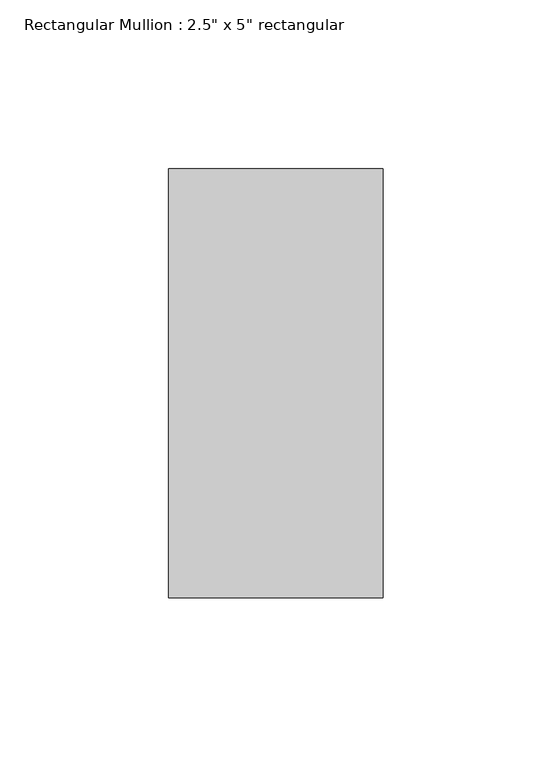
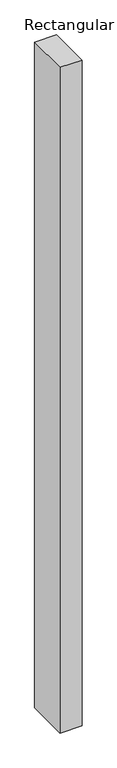
"""IFC4 building model written with IfcOpenShell, lengths in millimetres: member geometry."""

from ifc_helpers import new_model, si_unit, frame, origin, place, context, project, spatial, polyline, outline, extrude, source, transform, mapped, element, save


def member_0a82c195(model_context):
    return source(origin(), model_context, "Body", "SweptSolid", [
        extrude(outline(polyline([(0.0, 63.5), (0.0, -63.5), (-63.5, -63.5), (-63.5, 63.5), (0.0, 63.5)])), frame((0.0, 0.0, -2032.0), z_axis=(0.0, 0.0, 1.0), x_axis=(1.0, 0.0, 0.0)), (0.0, 0.0, 1.0), 2032.0),
    ])


if __name__ == "__main__":
    model = new_model("IFC4")
    model_context = context("Model", 3, world=origin())
    ifc_project = project(units=[si_unit("LENGTHUNIT", "METRE", prefix="MILLI")], contexts=[model_context])
    site = spatial("IfcSite", under=ifc_project)
    building = spatial("IfcBuilding", under=site)
    placement = place(None, origin())
    member_shape = member_0a82c195(model_context)
    element("IfcMember", 1, ObjectType="Rectangular Mullion : 2.5\" x 5\" rectangular", at=placement, inside=building, context=model_context, shape_type="MappedRepresentation", body=[
        mapped(member_shape, transform((0.0, 0.0, 0.0), x_axis=(1.0, 0.0, 0.0), y_axis=(0.0, 1.0, 0.0), z_axis=(0.0, 0.0, 1.0))),
    ])
    save(model, "model.ifc")

# Revit data of these elements
# Type "Rectangular Mullion : 2.5\" x 5\" rectangular"
#   built-in parameter 1007304 = 0.416667 (stored number, unit not read)
#   built-in parameter 1007301 = 0.104167 (stored number, unit not read)
#   built-in parameter 1007300 = 0.104167 (stored number, unit not read)
